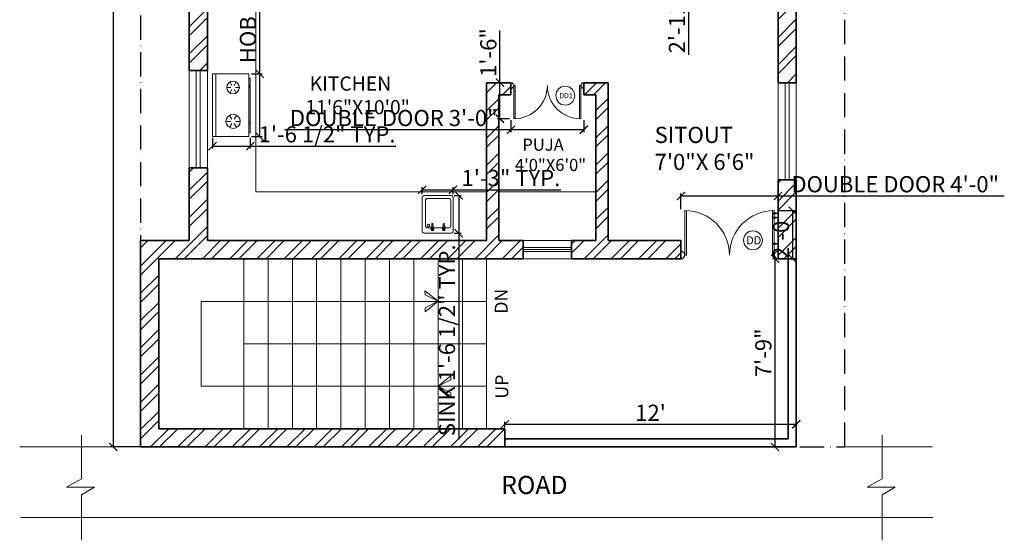
# Model space of a CAD drawing. Units: inches. Extents: x -15 to 1053, y -1 to 793.
# Tile 4 of 8: x 559 to 1046, y -1 to 256. Entities that reach past the tile are written whole.
import ezdxf

# ---------------------------------------------------------------- set-up
doc = ezdxf.new("R2010")
doc.units = ezdxf.units.IN
doc.linetypes.add('ACAD_ISO10W100', pattern=[18, 12, -3, 0, -3])
for name, color, linetype, lineweight in [('00 FURNITURE', 15, 'Continuous', 15), ('A-ANNO-DIMS', 2, 'Continuous', 18), ('A-ANNO-SYMB', 2, 'Continuous', 18), ('A-ANNO-TEXT', 7, 'Continuous', 18), ('A-AREA-IDEN', 7, 'Continuous', 18), ('A-DOOR', 4, 'Continuous', 18), ('A-FLOR-CASE', 5, 'Continuous', 18), ('A-FLOR-FIXT', 8, 'Continuous', 13), ('A-FLOR-STRS', 3, 'Continuous', 18), ('A-GLAZ', 4, 'Continuous', 18), ('A-WALL', 7, 'Continuous', 35), ('A-WALL-PATT', 8, 'Continuous', 13), ('C-PROP', 1, 'ACAD_ISO10W100', 25), ('C-ROAD', 7, 'Continuous', 18)]:
    doc.layers.add(name, color=color, linetype=linetype, lineweight=lineweight)
doc.layers.add('FURN3D', color=229, linetype='Continuous', lineweight=5, true_color=0x4a3f41)
doc.styles.add('1-100DIM', font='txt', dxfattribs={"height": 0.3})
doc.styles.get("Standard").update_dxf_attribs({"font": 'arial.ttf'})
doc.dimstyles.new('ISO-25', dxfattribs={"dimtxt": 8, "dimasz": 4, "dimexe": 1.25, "dimexo": 0.625, "dimtad": 1, "dimdec": 0, "dimlunit": 4, "dimtxsty": 'Standard', "dimblk": 'ARCHTICK', "dimcen": 3, "dimadec": 0, "dimazin": 0, "dimtfac": 1, "dimtdec": 0, "dimtmove": 0, "dimatfit": 3, "dimldrblk": 'ARCHTICK', "dimfxl": 1, "dimarcsym": 0})

# ---------------------------------------------------------------- blocks, each defined once
blk = doc.blocks.new('A$C03CC5C65')
at = {"layer": 'FURN3D'}
for p, q in [((0, 0.9, -49.92), (0, 17.82, -49.92)), ((0, 0.9, -29.27), (0, 17.82, -48.65)), ((0, 17.82, -29.27), (0, 0.9, -48.65)), ((1.56, 18.72, -49.92), (13.66, 18.72, -49.92)), ((4.37, 16.77, -25.9), (4.37, 16.84, -25.9)), ((4.37, 16.77, -25.9), (4.73, 16.4, -25.9)), ((4.37, 15.7, -25.9), (4.73, 16.12, -25.9)), ((4.37, 15.64, -25.9), (4.73, 16.06, -25.9)), ((4.37, 15.64, -25.9), (4.37, 15.7, -25.9)), ((4.48, 16.95, -25.9), (4.87, 16.59, -25.9)), ((4.48, 16.89, -25.9), (4.48, 16.95, -25.9)), ((4.48, 16.89, -25.9), (4.87, 16.52, -25.9)), ((4.48, 15.53, -25.9), (4.87, 15.89, -25.9)), ((4.63, 16.87, -25.9), (4.63, 16.8, -25.9)), ((4.63, 15.67, -25.9), (4.68, 15.67, -25.9)), ((4.63, 15.67), (4.68, 15.67)), ((4.64, 16.49, -25.9), (4.66, 16.05, -25.9)), ((4.83, 16.98, -25.9), (4.68, 16.76, -25.9)), ((4.68, 15.71, -25.9), (4.75, 14.17, -25.9)), ((4.87, 16.91, -25.9), (4.73, 16.71, -25.9)), ((5.24, 16.98, -25.9), (4.83, 16.98, -25.9)), ((4.87, 16.91, -25.9), (4.83, 16.98, -25.9)), ((5.21, 16.91, -25.9), (4.87, 16.91, -25.9)), ((5.21, 16.91, -25.9), (5.24, 16.98, -25.9)), ((5.6, 16.95, -25.9), (5.21, 16.59, -25.9)), ((5.21, 16.91, -25.9), (5.34, 16.71, -25.9)), ((5.6, 16.88, -25.9), (5.21, 16.52, -25.9)), ((5.6, 15.52, -25.9), (5.21, 15.89, -25.9)), ((5.24, 16.98, -25.9), (5.39, 16.76, -25.9)), ((5.39, 15.71, -25.9), (5.32, 14.17, -25.9)), ((5.71, 16.77, -25.9), (5.35, 16.4, -25.9)), ((5.71, 15.7, -25.9), (5.35, 16.12, -25.9)), ((5.71, 15.64, -25.9), (5.35, 16.06, -25.9)), ((5.39, 15.67, -25.9), (5.44, 15.67, -25.9)), ((5.39, 15.67), (5.44, 15.67)), ((5.43, 16.49, -25.9), (5.41, 16.05, -25.9)), ((5.44, 16.87, -25.9), (5.44, 16.8, -25.9)), ((5.6, 16.95, -25.9), (5.6, 16.88, -25.9)), ((5.6, 16.95, -25.9), (5.6, 16.88, -25.9)), ((5.71, 16.77, -25.9), (5.71, 16.83, -25.9)), ((5.71, 15.64, -25.9), (5.71, 15.7, -25.9)), ((9.98, 15.69, -25.9), (10.34, 16.11, -25.9)), ((9.98, 15.63, -25.9), (10.34, 16.05, -25.9)), ((9.98, 15.63, -25.9), (9.98, 15.69, -25.9)), ((9.99, 16.76, -25.9), (9.99, 16.83, -25.9)), ((9.99, 16.76, -25.9), (10.34, 16.39, -25.9)), ((10.09, 16.94, -25.9), (10.48, 16.58, -25.9)), ((10.09, 16.88, -25.9), (10.09, 16.94, -25.9)), ((10.09, 16.88, -25.9), (10.48, 16.51, -25.9)), ((10.09, 15.52, -25.9), (10.48, 15.88, -25.9)), ((10.25, 16.86, -25.9), (10.25, 16.8, -25.9)), ((10.25, 15.66, -25.9), (10.3, 15.66, -25.9)), ((10.25, 15.66), (10.3, 15.66)), ((10.26, 16.47, -25.9), (10.28, 16.03, -25.9)), ((10.45, 16.97, -25.9), (10.3, 16.75, -25.9)), ((10.3, 15.7, -25.9), (10.37, 14.16, -25.9)), ((10.49, 16.9, -25.9), (10.35, 16.7, -25.9)), ((10.86, 16.97, -25.9), (10.45, 16.97, -25.9)), ((10.49, 16.9, -25.9), (10.45, 16.97, -25.9)), ((10.82, 16.9, -25.9), (10.49, 16.9, -25.9)), ((10.82, 16.9, -25.9), (10.86, 16.97, -25.9)), ((11.22, 16.94, -25.9), (10.82, 16.58, -25.9)), ((10.82, 16.9, -25.9), (10.96, 16.7, -25.9)), ((11.22, 16.88, -25.9), (10.82, 16.51, -25.9)), ((11.21, 15.51, -25.9), (10.82, 15.88, -25.9)), ((10.86, 16.97, -25.9), (11.01, 16.75, -25.9)), ((11.01, 15.7, -25.9), (10.93, 14.16, -25.9)), ((11.32, 16.76, -25.9), (10.96, 16.39, -25.9)), ((11.32, 15.69, -25.9), (10.96, 16.11, -25.9)), ((11.32, 15.63, -25.9), (10.96, 16.05, -25.9)), ((11.01, 15.66, -25.9), (11.06, 15.66, -25.9)), ((11.01, 15.66), (11.06, 15.66)), ((11.05, 16.47, -25.9), (11.03, 16.03, -25.9)), ((11.06, 16.86, -25.9), (11.06, 16.8, -25.9)), ((11.22, 16.94, -25.9), (11.22, 16.88, -25.9)), ((11.22, 16.94, -25.9), (11.22, 16.88, -25.9)), ((11.32, 16.76, -25.9), (11.32, 16.83, -25.9)), ((11.32, 15.63, -25.9), (11.32, 15.69, -25.9)), ((15.22, 0.9, -29.27), (15.22, 17.82, -48.65)), ((15.22, 17.82, -29.27), (15.22, 0.9, -48.65)), ((1.56, 0, -28), (13.66, 0, -28))]:
    blk.add_line(p, q, dxfattribs=at)
at = {"layer": 'FURN3D', "elevation": -25.9}
for points in [[(1.61, 15.14), (1.62, 2.5)], [(4.66, 16.1), (2.57, 16.1)], [(10.28, 16.11), (5.41, 16.1)], [(13.12, 16.11), (11.03, 16.11)], [(14.1, 2.52), (14.09, 15.15)], [(2.58, 1.55), (13.13, 1.56)]]:
    blk.add_lwpolyline(points, dxfattribs=at)
at = {"layer": 'FURN3D'}
for centre, radius in [((3.1, 14.9, -25.9), 0.593), ((5.04, 16.22, -25.9), 0.218), ((5.04, 16.87), 0.203), ((5.04, 16.87, -25.9), 0.203), ((10.65, 16.22, -25.9), 0.218), ((10.65, 16.86), 0.203), ((10.65, 16.86, -25.9), 0.203)]:
    blk.add_circle(centre, radius, dxfattribs=at)
at = {"layer": 'FURN3D', "extrusion": (0, 0.814703, 0.579878)}
for centre, start, end in [((-1.56, -49.97, -13.7), 270, 0), ((-13.66, -49.97, -13.7), 180, 270), ((-1.56, -24.37, -16.24), 0, 90), ((-13.66, -24.37, -16.24), 90, 180)]:
    blk.add_arc(centre, 1.56, start, end, dxfattribs=at)
at = {"layer": 'FURN3D', "extrusion": (2.9e-15, -0.814703, 0.579878)}
for centre, start, end in [((1.56, -13.52, -31.49), 90, 180), ((1.56, -39.11, -28.95), 180, 270)]:
    blk.add_arc(centre, 1.56, start, end, dxfattribs=at)
at = {"layer": 'FURN3D'}
for centre, radius, start, end in [((2.6, 15.1, -25.9), 0.997, 88.2299, 182.3676), ((4.6, 16.73, -25.9), 0.252, 118.1078, 154.1122), ((4.6, 16.66, -25.9), 0.252, 118.1078, 154.1122), ((4.6, 15.75, -25.9), 0.252, 205.7141, 241.7184), ((5.04, 16.87, -25.9), 0.655, 359.2227, 180.6036), ((5.04, 16.88, -25.9), 0.655, 190.8582, 233.614), ((5.04, 16.87, -25.9), 0.406, 359.9131, 179.9131), ((4.54, 16.23, -25.9), 0.25, 317.2189, 42.6074), ((4.54, 16.29, -25.9), 0.25, 317.2189, 352.664), ((5.04, 16.6, -25.9), 0.312, 19.462, 160.6639), ((5.04, 16.24, -25.9), 0.218, 356.8132, 183.0131), ((5.04, 16.77, -25.9), 0.25, 227.2092, 312.6171), ((5.04, 16.71, -25.9), 0.25, 227.2092, 312.6171), ((5.04, 15.7, -25.9), 0.25, 47.2092, 132.6171), ((5.04, 16.44, -25.9), 0.187, 40.218, 139.6082), ((5.53, 16.23, -25.9), 0.25, 137.2189, 222.6074), ((5.53, 16.29, -25.9), 0.25, 187.1622, 222.6074), ((5.04, 16.88, -25.9), 0.655, 306.2123, 348.968), ((5.48, 16.72, -25.9), 0.252, 25.7141, 61.7184), ((5.48, 16.66, -25.9), 0.252, 25.7141, 61.7184), ((5.48, 15.75, -25.9), 0.252, 298.1078, 334.1122), ((10.21, 15.74, -25.9), 0.252, 205.7141, 241.7184), ((10.21, 16.72, -25.9), 0.252, 118.1078, 154.1122), ((10.21, 16.65, -25.9), 0.252, 118.1078, 154.1122), ((10.65, 16.86, -25.9), 0.655, 359.2227, 180.6036), ((10.65, 16.86, -25.9), 0.655, 190.8582, 233.614), ((10.65, 16.86, -25.9), 0.406, 359.9131, 179.9131), ((10.16, 16.22, -25.9), 0.25, 317.2189, 42.6074), ((10.16, 16.28, -25.9), 0.25, 317.2189, 352.664), ((10.66, 16.59, -25.9), 0.312, 19.462, 160.6639), ((10.65, 16.23, -25.9), 0.218, 356.8132, 183.0131), ((10.65, 16.7, -25.9), 0.25, 227.2092, 312.6171), ((10.65, 15.69, -25.9), 0.25, 47.2092, 132.6171), ((10.65, 16.76, -25.9), 0.25, 227.2092, 312.6171), ((10.65, 16.44, -25.9), 0.187, 40.218, 139.6082), ((11.15, 16.22, -25.9), 0.25, 137.2189, 222.6074), ((11.15, 16.28, -25.9), 0.25, 187.1622, 222.6074), ((10.65, 16.86, -25.9), 0.655, 306.2123, 348.968), ((11.1, 15.74, -25.9), 0.252, 298.1078, 334.1122), ((11.1, 16.72, -25.9), 0.252, 25.7141, 61.7184), ((11.1, 16.65, -25.9), 0.252, 25.7141, 61.7184), ((13.09, 15.11, -25.9), 0.997, 357.7426, 91.8802), ((5.04, 14.37, -25.9), 0.298, 194.8671, 343.5351), ((5.03, 14.18, -25.9), 0.281, 182.7661, 357.0602), ((10.65, 14.36, -25.9), 0.298, 194.8671, 343.5351), ((10.65, 14.17, -25.9), 0.281, 182.7661, 357.0602), ((2.61, 2.54, -25.9), 0.997, 177.7426, 271.8802), ((13.1, 2.55, -25.9), 0.997, 268.2299, 2.3676)]:
    blk.add_arc(centre, radius, start, end, dxfattribs=at)
at = {"layer": 'FURN3D', "extrusion": (-2.9e-15, -0.814703, 0.579878)}
for centre, start, end in [((13.66, -13.52, -31.49), 0, 90), ((13.66, -39.11, -28.95), 270, 0)]:
    blk.add_arc(centre, 1.56, start, end, dxfattribs=at)
blk = doc.blocks.new('_ArchTick')
at = {"color": 0, "linetype": 'ByBlock', "const_width": 0.15}
blk.add_lwpolyline([(-0.5, -0.5), (0.5, 0.5)], dxfattribs=at)
blk = doc.blocks.new('*D19')
at = {"layer": 'A-ANNO-DIMS', "color": 0, "lineweight": -2, "transparency": 16777216}
for p, q in [((618.45, 764.76), (604.32, 764.76)), ((605.57, 764.76), (605.57, 44.76)), ((618.45, 44.76), (604.32, 44.76))]:
    blk.add_line(p, q, dxfattribs=at)
at = {"layer": 'Defpoints', "color": 0, "transparency": 16777216}
for p in [(619.07, 764.76), (605.57, 44.76), (619.07, 44.76)]:
    blk.add_point(p, dxfattribs=at)
at = {"layer": 'A-ANNO-DIMS', "color": 0, "lineweight": -2, "transparency": 16777216, "xscale": 4, "yscale": 4, "zscale": 4}
for p, rotation in [((605.57, 764.76), 90), ((605.57, 44.76), 270)]:
    blk.add_blockref('_ArchTick', p, dxfattribs=dict(at, rotation=rotation))
at = {"layer": 'A-ANNO-DIMS', "color": 0, "transparency": 16777216, "insert": (600.86, 404.76), "char_height": 8, "attachment_point": 5, "rotation": 90}
blk.add_mtext("60'", dxfattribs=at)
blk = doc.blocks.new('A$C21540130')
at = {"layer": 'FURN3D'}
for p, q in [((1.57, 0), (1.57, 31.11)), ((9.61, 25.31), (8.63, 27.01)), ((10.79, 25.31), (11.77, 27.01)), ((9.02, 24.29, -27.54), (7.06, 24.29, -27.54)), ((9.61, 23.27), (8.63, 21.57)), ((10.79, 23.27), (11.77, 21.57)), ((11.38, 24.29, -27.54), (13.34, 24.29, -27.54)), ((9.61, 8.56), (8.43, 10.6)), ((10.79, 8.56), (11.97, 10.6)), ((9.02, 7.54), (6.67, 7.54)), ((9.61, 6.52), (8.43, 4.48)), ((10.79, 6.52), (11.97, 4.48)), ((11.38, 7.54), (13.73, 7.54))]:
    blk.add_line(p, q, dxfattribs=at)
for points in [[(0, 0), (0, 31.11), (17.9, 31.11), (17.9, 0)], [(18.68, 1.96), (18.68, 28.83), (17.9, 28.83), (17.9, 1.96)]]:
    blk.add_lwpolyline(points, close=True, dxfattribs=at)
for centre, radius in [((10.2, 24.29), 3.14), ((10.2, 7.54), 3.53)]:
    blk.add_circle(centre, radius, dxfattribs=at)
for points in [[(17.9, 24.03), (18.29, 24.03), (17.9, 25.6), (18.29, 25.6)], [(17.9, 6.05), (18.29, 6.05), (17.9, 7.62), (18.29, 7.62)]]:
    blk.add_solid(points, dxfattribs=at)
blk = doc.blocks.new('PUJA')
at = {"layer": '00 FURNITURE'}
for p, q in [((-1940.35, -16093.35), (-1958.14, -16093.35)), ((-1940.35, -16093.93), (-1958.13, -16093.93)), ((-1941.8, -16091.75), (-1938.89, -16091.75)), ((-1941.8, -16092.33), (-1941.8, -16091.75)), ((-1941.22, -16092.62), (-1941.51, -16092.62)), ((-1940.35, -16093.35), (-1940.35, -16093.93)), ((-1939.18, -16092.62), (-1939.47, -16092.62)), ((-1938.89, -16091.75), (-1938.89, -16092.33)), ((-1940.35, -16128.93), (-1958.14, -16128.93)), ((-1940.35, -16128.35), (-1958.13, -16128.35)), ((-1941.8, -16129.96), (-1941.8, -16130.54)), ((-1941.22, -16129.66), (-1941.51, -16129.66)), ((-1940.35, -16128.93), (-1940.35, -16128.35)), ((-1939.18, -16129.66), (-1939.47, -16129.66)), ((-1938.89, -16130.54), (-1938.89, -16129.96)), ((-1941.8, -16130.54), (-1938.89, -16130.54))]:
    blk.add_line(p, q, dxfattribs=at)
for points in [[(-1939.47, -16092.62), (-1939.47, -16092.91, -0.414214), (-1939.76, -16093.21), (-1940.93, -16093.21, -0.414214), (-1941.22, -16092.91), (-1941.22, -16092.62)], [(-1939.47, -16129.66), (-1939.47, -16129.37, 0.414214), (-1939.76, -16129.08), (-1940.93, -16129.08, 0.414214), (-1941.22, -16129.37), (-1941.22, -16129.66)]]:
    blk.add_lwpolyline(points, format="xyb", dxfattribs=at)
for centre, radius, start, end in [((-1940.35, -16093.35), 17.79, 180, 270), ((-1941.51, -16092.33), 0.292, 180, 270), ((-1939.18, -16092.33), 0.292, 270, 0), ((-1940.35, -16128.93), 17.79, 90, 180), ((-1941.51, -16129.96), 0.292, 90, 180), ((-1939.18, -16129.96), 0.292, 0, 90)]:
    blk.add_arc(centre, radius, start, end, dxfattribs=at)
blk = doc.blocks.new('*D28')
at = {"layer": 'A-ANNO-DIMS', "color": 0, "lineweight": -2, "transparency": 16777216}
for p, q in [((799.07, 54.39), (799.07, 57.2)), ((799.07, 55.95), (943.07, 55.95)), ((943.07, 45.39), (943.07, 57.2))]:
    blk.add_line(p, q, dxfattribs=at)
at = {"layer": 'Defpoints', "color": 0, "transparency": 16777216}
for p in [(799.07, 53.76), (943.07, 55.95), (943.07, 44.76)]:
    blk.add_point(p, dxfattribs=at)
at = {"layer": 'A-ANNO-DIMS', "color": 0, "lineweight": -2, "transparency": 16777216, "xscale": 4, "yscale": 4, "zscale": 4, "rotation": 180}
blk.add_blockref('_ArchTick', (799.07, 55.95), dxfattribs=at)
at = {"layer": 'A-ANNO-DIMS', "color": 0, "lineweight": -2, "transparency": 16777216, "xscale": 4, "yscale": 4, "zscale": 4}
blk.add_blockref('_ArchTick', (943.07, 55.95), dxfattribs=at)
at = {"layer": 'A-ANNO-DIMS', "color": 0, "transparency": 16777216, "insert": (871.07, 60.59), "char_height": 8, "attachment_point": 5}
blk.add_mtext("12'", dxfattribs=at)
blk = doc.blocks.new('*D29')
at = {"layer": 'A-ANNO-DIMS', "color": 0, "lineweight": -2, "transparency": 16777216}
for p, q in [((942.45, 137.76), (931.3, 137.76)), ((932.55, 137.76), (932.55, 44.76)), ((942.45, 44.76), (931.3, 44.76))]:
    blk.add_line(p, q, dxfattribs=at)
at = {"layer": 'Defpoints', "color": 0, "transparency": 16777216}
for p in [(943.07, 137.76), (932.55, 44.76), (943.07, 44.76)]:
    blk.add_point(p, dxfattribs=at)
at = {"layer": 'A-ANNO-DIMS', "color": 0, "lineweight": -2, "transparency": 16777216, "xscale": 4, "yscale": 4, "zscale": 4}
for p, rotation in [((932.55, 137.76), 90), ((932.55, 44.76), 270)]:
    blk.add_blockref('_ArchTick', p, dxfattribs=dict(at, rotation=rotation))
at = {"layer": 'A-ANNO-DIMS', "color": 0, "transparency": 16777216, "insert": (927.84, 91.26), "char_height": 8, "attachment_point": 5, "rotation": 90}
blk.add_mtext('7\'-9"', dxfattribs=at)
blk = doc.blocks.new('BREAK-SYMBOL')
for p, q in [((7.31, 51.97), (7.31, 30.42)), ((7.31, 30.42), (0, 26.2)), ((0, 26.2), (13.84, 26.2)), ((13.84, 26.2), (7.31, 22.43)), ((7.31, 22.43), (7.31, 0))]:
    blk.add_line(p, q)
blk = doc.blocks.new('*D47')
at = {"layer": 'A-ANNO-DIMS', "color": 0, "lineweight": -2, "transparency": 16777216}
for p, q in [((894.42, 333.87), (888.54, 333.87)), ((889.79, 333.87), (889.79, 298.84)), ((894.42, 298.84), (888.54, 298.84)), ((889.79, 298.84), (889.79, 238.47))]:
    blk.add_line(p, q, dxfattribs=at)
at = {"layer": 'Defpoints', "color": 0, "transparency": 16777216}
for p in [(895.05, 333.87), (889.79, 298.84), (895.05, 298.84)]:
    blk.add_point(p, dxfattribs=at)
at = {"layer": 'A-ANNO-DIMS', "color": 0, "lineweight": -2, "transparency": 16777216, "xscale": 4, "yscale": 4, "zscale": 4}
for p, rotation in [((889.79, 333.87), 90), ((889.79, 298.84), 270)]:
    blk.add_blockref('_ArchTick', p, dxfattribs=dict(at, rotation=rotation))
at = {"layer": 'A-ANNO-DIMS', "color": 0, "transparency": 16777216, "insert": (885.15, 266.65), "char_height": 8, "attachment_point": 5, "rotation": 90}
blk.add_mtext('2\'-11" TYP.', dxfattribs=at)
blk = doc.blocks.new('*D48')
at = {"layer": 'A-ANNO-DIMS', "color": 0, "lineweight": -2, "transparency": 16777216}
for p, q in [((774.07, 169.08), (777.51, 169.08)), ((776.26, 169.08), (776.26, 150.36)), ((774.07, 150.36), (777.51, 150.36)), ((776.26, 150.36), (776.26, 48.55))]:
    blk.add_line(p, q, dxfattribs=at)
at = {"layer": 'Defpoints', "color": 0, "transparency": 16777216}
for p in [(773.45, 169.08), (773.45, 150.36), (776.26, 150.36)]:
    blk.add_point(p, dxfattribs=at)
at = {"layer": 'A-ANNO-DIMS', "color": 0, "lineweight": -2, "transparency": 16777216, "xscale": 4, "yscale": 4, "zscale": 4}
for p, rotation in [((776.26, 169.08), 90), ((776.26, 150.36), 270)]:
    blk.add_blockref('_ArchTick', p, dxfattribs=dict(at, rotation=rotation))
at = {"layer": 'A-ANNO-DIMS', "color": 0, "transparency": 16777216, "insert": (771.5, 97.45), "char_height": 8, "attachment_point": 5, "rotation": 90}
blk.add_mtext('SINK 1\'-6 1/2" TYP.', dxfattribs=at)
blk = doc.blocks.new('*D49')
at = {"layer": 'A-ANNO-DIMS', "color": 0, "lineweight": -2, "transparency": 16777216}
for p, q in [((758.23, 169.7), (758.23, 173.13)), ((758.23, 171.88), (773.45, 171.88)), ((773.45, 169.7), (773.45, 173.13)), ((773.45, 171.88), (826.71, 171.88))]:
    blk.add_line(p, q, dxfattribs=at)
at = {"layer": 'Defpoints', "color": 0, "transparency": 16777216}
for p in [(773.45, 171.88), (758.23, 169.08), (773.45, 169.08)]:
    blk.add_point(p, dxfattribs=at)
at = {"layer": 'A-ANNO-DIMS', "color": 0, "lineweight": -2, "transparency": 16777216, "xscale": 4, "yscale": 4, "zscale": 4, "rotation": 180}
blk.add_blockref('_ArchTick', (758.23, 171.88), dxfattribs=at)
at = {"layer": 'A-ANNO-DIMS', "color": 0, "lineweight": -2, "transparency": 16777216, "xscale": 4, "yscale": 4, "zscale": 4}
blk.add_blockref('_ArchTick', (773.45, 171.88), dxfattribs=at)
at = {"layer": 'A-ANNO-DIMS', "color": 0, "transparency": 16777216, "insert": (802.08, 176.6), "char_height": 8, "attachment_point": 5}
blk.add_mtext('1\'-3" TYP.', dxfattribs=at)
blk = doc.blocks.new('*D50')
at = {"layer": 'A-ANNO-DIMS', "color": 0, "lineweight": -2, "transparency": 16777216}
for p, q in [((677.95, 229.2), (677.95, 310.11)), ((673.9, 229.2), (679.2, 229.2)), ((677.95, 198.09), (677.95, 229.2)), ((673.9, 198.09), (679.2, 198.09))]:
    blk.add_line(p, q, dxfattribs=at)
at = {"layer": 'Defpoints', "color": 0, "transparency": 16777216}
for p in [(673.28, 229.2), (677.95, 229.2), (673.28, 198.09)]:
    blk.add_point(p, dxfattribs=at)
at = {"layer": 'A-ANNO-DIMS', "color": 0, "lineweight": -2, "transparency": 16777216, "xscale": 4, "yscale": 4, "zscale": 4}
for p, rotation in [((677.95, 229.2), 90), ((677.95, 198.09), 270)]:
    blk.add_blockref('_ArchTick', p, dxfattribs=dict(at, rotation=rotation))
at = {"layer": 'A-ANNO-DIMS', "color": 0, "transparency": 16777216, "insert": (673.18, 271.65), "char_height": 8, "attachment_point": 5, "rotation": 90}
blk.add_mtext('HOB 2\'-7" TYP.', dxfattribs=at)
blk = doc.blocks.new('*D51')
at = {"layer": 'A-ANNO-DIMS', "color": 0, "lineweight": -2, "transparency": 16777216}
for p, q in [((654.6, 197.47), (654.6, 192.18)), ((673.28, 197.47), (673.28, 192.18)), ((654.6, 193.43), (673.28, 193.43)), ((673.28, 193.43), (745.18, 193.43))]:
    blk.add_line(p, q, dxfattribs=at)
at = {"layer": 'Defpoints', "color": 0, "transparency": 16777216}
for p in [(654.6, 198.09), (673.28, 198.09), (673.28, 193.43)]:
    blk.add_point(p, dxfattribs=at)
at = {"layer": 'A-ANNO-DIMS', "color": 0, "lineweight": -2, "transparency": 16777216, "xscale": 4, "yscale": 4, "zscale": 4, "rotation": 180}
blk.add_blockref('_ArchTick', (654.6, 193.43), dxfattribs=at)
at = {"layer": 'A-ANNO-DIMS', "color": 0, "lineweight": -2, "transparency": 16777216, "xscale": 4, "yscale": 4, "zscale": 4}
blk.add_blockref('_ArchTick', (673.28, 193.43), dxfattribs=at)
at = {"layer": 'A-ANNO-DIMS', "color": 0, "transparency": 16777216, "insert": (711.23, 198.19), "char_height": 8, "attachment_point": 5}
blk.add_mtext('1\'-6 1/2" TYP.', dxfattribs=at)
blk = doc.blocks.new('*D54')
at = {"layer": 'A-ANNO-DIMS', "color": 0, "lineweight": -2, "transparency": 16777216}
for p, q in [((886.07, 162.21), (886.07, 170.03)), ((886.07, 168.78), (934.07, 168.78)), ((934.07, 162.21), (934.07, 170.03)), ((934.07, 168.78), (1045.89, 168.78))]:
    blk.add_line(p, q, dxfattribs=at)
at = {"layer": 'Defpoints', "color": 0, "transparency": 16777216}
for p in [(934.07, 168.78), (886.07, 161.58), (934.07, 161.58)]:
    blk.add_point(p, dxfattribs=at)
at = {"layer": 'A-ANNO-DIMS', "color": 0, "lineweight": -2, "transparency": 16777216, "xscale": 4, "yscale": 4, "zscale": 4, "rotation": 180}
blk.add_blockref('_ArchTick', (886.07, 168.78), dxfattribs=at)
at = {"layer": 'A-ANNO-DIMS', "color": 0, "lineweight": -2, "transparency": 16777216, "xscale": 4, "yscale": 4, "zscale": 4}
blk.add_blockref('_ArchTick', (934.07, 168.78), dxfattribs=at)
at = {"layer": 'A-ANNO-DIMS', "color": 0, "transparency": 16777216, "insert": (991.98, 173.55), "char_height": 8, "attachment_point": 5}
blk.add_mtext('DOUBLE DOOR 4\'-0"', dxfattribs=at)
blk = doc.blocks.new('*D55')
at = {"layer": 'A-ANNO-DIMS', "color": 0, "lineweight": -2, "transparency": 16777216}
for p, q in [((934.7, 161.58), (942.52, 161.58)), ((941.27, 161.58), (941.27, 137.76)), ((934.7, 137.76), (942.52, 137.76))]:
    blk.add_line(p, q, dxfattribs=at)
at = {"layer": 'Defpoints', "color": 0, "transparency": 16777216}
for p in [(934.07, 161.58), (934.07, 137.76), (941.27, 137.76)]:
    blk.add_point(p, dxfattribs=at)
at = {"layer": 'A-ANNO-DIMS', "color": 0, "lineweight": -2, "transparency": 16777216, "xscale": 4, "yscale": 4, "zscale": 4}
for p, rotation in [((941.27, 161.58), 90), ((941.27, 137.76), 270)]:
    blk.add_blockref('_ArchTick', p, dxfattribs=dict(at, rotation=rotation))
at = {"layer": 'A-ANNO-DIMS', "color": 0, "transparency": 16777216, "insert": (936.56, 149.67), "char_height": 8, "attachment_point": 5, "rotation": 90}
blk.add_mtext('2\'-0"', dxfattribs=at)
blk = doc.blocks.new('*D56')
at = {"layer": 'A-ANNO-DIMS', "color": 0, "lineweight": -2, "transparency": 16777216}
for p, q in [((802.07, 206.27), (802.07, 200.25)), ((838.07, 206.27), (838.07, 200.25)), ((802.07, 201.5), (690.26, 201.5)), ((838.07, 201.5), (802.07, 201.5))]:
    blk.add_line(p, q, dxfattribs=at)
at = {"layer": 'Defpoints', "color": 0, "transparency": 16777216}
for p in [(802.07, 206.9), (838.07, 206.9), (802.07, 201.5)]:
    blk.add_point(p, dxfattribs=at)
at = {"layer": 'A-ANNO-DIMS', "color": 0, "lineweight": -2, "transparency": 16777216, "xscale": 4, "yscale": 4, "zscale": 4}
for p, rotation in [((802.07, 201.5), 180.0000000034012), ((838.07, 201.5), 3.4012793e-09)]:
    blk.add_blockref('_ArchTick', p, dxfattribs=dict(at, rotation=rotation))
at = {"layer": 'A-ANNO-DIMS', "color": 0, "transparency": 16777216, "insert": (744.17, 206.27), "char_height": 8, "attachment_point": 5, "rotation": 0}
blk.add_mtext('DOUBLE DOOR 3\'-0"', dxfattribs=at)
blk = doc.blocks.new('*D57')
at = {"layer": 'A-ANNO-DIMS', "color": 0, "lineweight": -2, "transparency": 16777216}
for p, q in [((796.67, 224.76), (796.67, 250.53)), ((801.45, 224.76), (795.42, 224.76)), ((796.67, 206.9), (796.67, 224.76)), ((801.45, 206.9), (795.42, 206.9))]:
    blk.add_line(p, q, dxfattribs=at)
at = {"layer": 'Defpoints', "color": 0, "transparency": 16777216}
for p in [(796.67, 224.76), (802.07, 224.76), (802.07, 206.9)]:
    blk.add_point(p, dxfattribs=at)
at = {"layer": 'A-ANNO-DIMS', "color": 0, "lineweight": -2, "transparency": 16777216, "xscale": 4, "yscale": 4, "zscale": 4}
for p, rotation in [((796.67, 224.76), 90), ((796.67, 206.9), 270)]:
    blk.add_blockref('_ArchTick', p, dxfattribs=dict(at, rotation=rotation))
at = {"layer": 'A-ANNO-DIMS', "color": 0, "transparency": 16777216, "insert": (791.96, 239.65), "char_height": 8, "attachment_point": 5, "rotation": 90}
blk.add_mtext('1\'-6"', dxfattribs=at)

msp = doc.modelspace()

# ---------------------------------------------------------------- hatches: boundary and pattern name
at = {"layer": 'A-WALL-PATT'}
h = msp.add_hatch(dxfattribs=at)
h.set_pattern_fill('ANSI32', color=256)
h.paths.add_polyline_path([(754.07, 502.76), (754.07, 503.76), (652.07, 503.76), (652.07, 593.76), (643.07, 593.76), (643.07, 485.76), (652.07, 485.76), (652.07, 497.76), (754.07, 497.76)])
h.paths.add_polyline_path([(754.07, 449.76), (730.07, 449.76), (730.07, 467.76), (724.07, 467.76), (724.07, 449.76), (652.07, 449.76), (652.07, 461.76), (643.07, 461.76), (643.07, 374.76), (652.07, 374.76), (652.07, 443.76), (754.07, 443.76)])
h.paths.add_polyline_path([(757.07, 740.76), (643.07, 740.76), (643.07, 641.76), (652.07, 641.76), (652.07, 731.76), (700.07, 731.76), (700.07, 701.76), (706.07, 701.76), (706.07, 731.76), (757.07, 731.76)])
h.paths.add_polyline_path([(943.07, 740.76), (781.07, 740.76), (781.07, 731.76), (790.07, 731.76), (790.07, 671.76), (688.07, 671.76), (688.07, 665.76), (790.07, 665.76), (790.07, 497.76), (796.07, 497.76), (796.07, 502.76), (796.07, 731.76), (844.07, 731.76), (844.07, 701.76), (850.07, 701.76), (850.07, 731.76), (934.07, 731.76), (934.07, 713.76), (943.07, 713.76)])
h.paths.add_polyline_path([(943.07, 689.76), (934.07, 689.76), (934.07, 671.76), (832.07, 671.76), (832.07, 665.76), (934.07, 665.76), (934.07, 608.76), (943.07, 608.76)], flags=17)
h.paths.add_polyline_path([(943.07, 560.76), (934.07, 560.76), (934.07, 503.76), (832.07, 503.76), (832.07, 497.76), (934.07, 497.76), (934.07, 488.76), (943.07, 488.76)])
h.paths.add_polyline_path([(796.07, 449.76), (790.07, 449.76), (790.07, 444.76), (790.07, 326.76), (643.07, 326.76), (643.07, 320.76), (724.07, 320.76), (724.07, 266.76), (730.07, 266.76), (730.07, 320.76), (790.07, 320.76), (790.07, 272.76), (760.07, 272.76), (760.07, 266.76), (796.07, 266.76)])
h.paths.add_polyline_path([(652.07, 266.76), (688.07, 266.76), (688.07, 271.76), (688.07, 272.76), (643.07, 272.76), (643.07, 230.76), (652.07, 230.76)])
h.paths.add_polyline_path([(652.07, 182.76), (643.07, 182.76), (643.07, 146.76), (619.07, 146.76), (619.07, 44.76), (799.07, 44.76), (799.07, 53.76), (628.07, 53.76), (628.07, 137.76), (808.07, 137.76), (808.07, 146.76), (796.07, 146.76), (796.07, 218.76), (802.07, 218.76), (802.07, 224.76), (790.07, 224.76), (790.07, 146.76), (652.07, 146.76)])
h.paths.add_polyline_path([(886.07, 141.37), (886.07, 146.76), (850.07, 146.76), (850.07, 224.76), (838.07, 224.76), (838.07, 222.06), (838.07, 218.76), (844.07, 218.76), (844.07, 146.76), (832.07, 146.76), (832.07, 137.76), (886.07, 137.76)])
h.paths.add_polyline_path([(943.07, 176.76), (934.07, 176.76), (934.07, 137.76), (943.07, 137.76)])
h.paths.add_polyline_path([(943.07, 440.76), (934.07, 440.76), (934.07, 224.76), (943.07, 224.76)])

# ---------------------------------------------------------------- linework, layer by layer
at = {"layer": 'A-ANNO-TEXT'}
for centre in [(828.93, 218.35), (921.67, 146.87)]:
    msp.add_circle(centre, 4.67, dxfattribs=at)
at = {"layer": 'A-FLOR-CASE'}
for p, q in [((676.07, 266.76), (676.07, 170.76)), ((676.07, 170.76), (790.07, 170.76)), ((796.07, 170.76), (844.07, 170.76))]:
    msp.add_line(p, q, dxfattribs=at)
at = {"layer": 'A-FLOR-STRS'}
for p, q in [((670.07, 137.76), (670.07, 53.76)), ((682.07, 137.76), (682.07, 53.76)), ((694.07, 137.76), (694.07, 53.76)), ((706.07, 137.76), (706.07, 53.76)), ((718.07, 137.76), (718.07, 53.76)), ((730.07, 137.76), (730.07, 53.76)), ((742.07, 137.76), (742.07, 53.76)), ((754.07, 137.76), (754.07, 53.76)), ((766.07, 137.76), (766.07, 53.76)), ((778.07, 137.76), (778.07, 53.76)), ((790.07, 137.76), (790.07, 53.76)), ((670.07, 95.76), (790.07, 95.76)), ((766.07, 74.76), (772.46, 69.56)), ((772.46, 71.55), (766.07, 74.76)), ((772.46, 69.56), (772.46, 71.55))]:
    msp.add_line(p, q, dxfattribs=at)
for points in [[(759.64, 119.88), (766.07, 116.76), (759.61, 121.87)], [(759.74, 113.46), (766.07, 116.76), (759.76, 111.47)], [(772.46, 79.96), (772.46, 77.97), (766.07, 74.76)]]:
    msp.add_lwpolyline(points, close=True, dxfattribs=at)
msp.add_lwpolyline([(790.07, 74.76), (649.07, 74.76), (649.07, 116.7), (790.07, 116.7)], dxfattribs=at)
at = {"layer": 'A-GLAZ'}
for p, q in [((643.07, 230.76), (643.07, 182.76)), ((646.57, 230.76), (646.57, 182.76)), ((648.57, 230.76), (648.57, 182.76)), ((652.07, 230.76), (652.07, 182.76)), ((934.07, 224.76), (934.07, 176.76)), ((937.57, 224.76), (937.57, 176.76)), ((939.57, 224.76), (939.57, 176.76)), ((943.07, 224.76), (943.07, 176.76)), ((832.07, 143.26), (808.07, 143.26)), ((832.07, 142.26), (808.07, 142.26)), ((832.07, 141.26), (808.07, 141.26))]:
    msp.add_line(p, q, dxfattribs=at)
msp.add_lwpolyline([(808.07, 146.76), (808.07, 137.76), (832.07, 137.76), (832.07, 146.76)], close=True, dxfattribs=at)
at = {"layer": 'A-WALL'}
for p, q in [((934.07, 224.76), (934.07, 440.76)), ((943.07, 224.76), (943.07, 440.76)), ((643.07, 272.76), (643.07, 230.76)), ((652.07, 266.76), (652.07, 230.76)), ((652.07, 230.76), (643.07, 230.76)), ((790.07, 224.76), (802.07, 224.76)), ((790.07, 224.76), (790.07, 146.76)), ((802.07, 218.76), (802.07, 224.76)), ((838.07, 218.76), (838.07, 224.76)), ((838.07, 224.76), (850.07, 224.76)), ((850.07, 224.76), (850.07, 146.76)), ((934.07, 224.76), (943.07, 224.76)), ((796.07, 218.76), (802.07, 218.76)), ((796.07, 218.76), (796.07, 146.76)), ((838.07, 218.76), (844.07, 218.76)), ((844.07, 218.76), (844.07, 146.76)), ((652.07, 182.76), (643.07, 182.76)), ((643.07, 182.76), (643.07, 146.76)), ((652.07, 182.76), (652.07, 146.76)), ((934.07, 137.76), (934.07, 176.76)), ((934.07, 176.76), (943.07, 176.76)), ((943.07, 137.76), (943.07, 176.76)), ((619.07, 146.76), (643.07, 146.76)), ((619.07, 146.76), (619.07, 44.76)), ((652.07, 146.76), (790.07, 146.76)), ((796.07, 146.76), (808.07, 146.76)), ((808.07, 146.76), (808.07, 137.76)), ((832.07, 146.76), (832.07, 137.76)), ((832.07, 146.76), (844.07, 146.76)), ((850.07, 146.76), (886.07, 146.76)), ((886.07, 137.76), (886.07, 146.76)), ((628.07, 137.76), (808.07, 137.76)), ((628.07, 137.76), (628.07, 53.76)), ((832.07, 137.76), (886.07, 137.76)), ((934.07, 137.76), (943.07, 137.76)), ((939.07, 137.76), (939.07, 48.76)), ((943.07, 137.76), (943.07, 44.76)), ((628.07, 53.76), (799.07, 53.76)), ((799.07, 53.76), (799.07, 44.76)), ((799.07, 48.76), (939.07, 48.76)), ((619.07, 44.76), (799.07, 44.76)), ((799.07, 44.76), (943.07, 44.76))]:
    msp.add_line(p, q, dxfattribs=at)
at = {"layer": 'C-PROP'}
for p, q in [((619.07, 764.76), (619.07, 44.76)), ((967.07, 44.76), (967.07, 764.76)), ((619.07, 44.76), (967.07, 44.76))]:
    msp.add_line(p, q, dxfattribs=at)
at = {"layer": 'C-ROAD'}
for p, q in [((619.07, 44.76), (559.32, 44.76)), ((967.07, 44.76), (1010.42, 44.76)), ((559.95, 9.83), (1010.56, 9.83))]:
    msp.add_line(p, q, dxfattribs=at)

# ---------------------------------------------------------------- block references
at = {"layer": 'A-ANNO-SYMB'}
for p in [(582.51, -1.39), (978.17, -1.39)]:
    msp.add_blockref('BREAK-SYMBOL', p, dxfattribs=at)
at = {"layer": 'A-DOOR'}
for p, xscale, yscale, zscale, rotation in [((-14131.62, 2024.12), 0.928034371616032, 0.928034371616032, 0.928034371616032, 90.00000000340147), ((20845.67, -2261.38), 1.237379162154587, 1.237379162154587, 1.237379162154587, 270.0000000034012)]:
    msp.add_blockref('PUJA', p, dxfattribs=dict(at, xscale=xscale, yscale=yscale, zscale=zscale, rotation=rotation))
at = {"layer": 'A-FLOR-FIXT'}
msp.add_blockref('A$C21540130', (654.6, 198.09), dxfattribs=at)
at = {"layer": 'A-FLOR-FIXT', "xscale": -1, "rotation": 180}
msp.add_blockref('A$C03CC5C65', (758.23, 169.08, 49.92), dxfattribs=at)

# ---------------------------------------------------------------- texts
at = {"layer": 'A-ANNO-TEXT', "attachment_point": 1}
for s, width, insert, char_height in [('DD1', 8.4888, (825.99, 219.6), 2.5), ('DD', 8.4888, (918.29, 148.88), 4), ('ROAD', 36.3273, (797.25, 30.45), 9)]:
    msp.add_mtext_dynamic_manual_height_columns(s, width=width, gutter_width=12.5, heights=[0], dxfattribs=dict(at, insert=insert, char_height=char_height))
at = {"layer": 'A-ANNO-TEXT', "char_height": 6.4099, "attachment_point": 3, "rotation": 90, "style": '1-100DIM'}
for s, insert in [('\\pxqc;{\\f@Malgun Gothic|b0|i0|c0|p34;DN}', (794.06, 139.01)), ('\\pxqc;{\\f@Malgun Gothic|b0|i0|c0|p34;UP}', (794.35, 96.8))]:
    msp.add_mtext_dynamic_manual_height_columns(s, width=44.4859, gutter_width=15.85, heights=[0], dxfattribs=dict(at, insert=insert))
at = {"layer": 'A-AREA-IDEN', "insert": (696.22, 227.83), "char_height": 7, "attachment_point": 1, "style": '1-100DIM'}
msp.add_mtext_dynamic_manual_height_columns('{\\f@Malgun Gothic|b0|i0|c0|p34;   KITCHEN\\P  11\'6"X10\'0"}', width=99.7063, gutter_width=15.85, heights=[0], dxfattribs=at)
at = {"layer": 'A-AREA-IDEN', "attachment_point": 1}
for s, width, heights, insert, char_height in [('  SITOUT\\P  7\'0"X 6\'6"', 62.9334, [0], (868.19, 202.95), 8), ('      PUJA       \\P    4\'0"X6\'0"', 44.0107, [18.97], (796.73, 197.11), 6)]:
    msp.add_mtext_dynamic_manual_height_columns(s, width=width, gutter_width=12.5, heights=heights, dxfattribs=dict(at, insert=insert, char_height=char_height))

# ---------------------------------------------------------------- dimensions: what is measured, and where the dimension line sits
at = {"layer": 'A-ANNO-DIMS'}
for base, p1, p2, angle, override, picture, middle in [((605.57, 44.76), (619.07, 764.76), (619.07, 44.76), 90, {"dimclrd": 0, "dimclre": 0, "dimclrt": 0}, '*D19', (600.86, 404.76)), ((796.67, 224.76), (802.07, 206.9), (802.07, 224.76), 90, {"dimdec": 1, "dimrnd": 0, "dimzin": 1, "dimlunit": 4, "dimfrac": 2}, '*D57', (791.96, 239.65)), ((941.27, 137.76), (934.07, 161.58), (934.07, 137.76), 270, {"dimdec": 1, "dimrnd": 0, "dimzin": 1, "dimlunit": 4, "dimfrac": 2}, '*D55', (936.56, 149.67)), ((932.55, 44.76), (943.07, 137.76), (943.07, 44.76), 90, {"dimclrd": 0, "dimclre": 0, "dimclrt": 0}, '*D29', (927.84, 91.26))]:
    dim = msp.add_linear_dim(base=base, p1=p1, p2=p2, angle=angle, dimstyle='ISO-25', override=override, dxfattribs=at)
    dim.commit()
    dim.dimension.update_dxf_attribs({"geometry": picture, "text_midpoint": middle})
for base, p1, p2, angle, text, picture, middle in [((889.79, 298.84), (895.05, 333.87), (895.05, 298.84), 270, '<> TYP.', '*D47', (885.15, 266.65)), ((677.95, 229.2), (673.28, 198.09), (673.28, 229.2), 90, 'HOB <> TYP.', '*D50', (673.18, 271.65)), ((802.07, 201.5), (838.07, 206.9), (802.07, 206.9), 180, 'DOUBLE DOOR <>', '*D56', (744.17, 206.27)), ((934.07, 168.78), (886.07, 161.58), (934.07, 161.58), 0, 'DOUBLE DOOR <>', '*D54', (991.98, 173.55)), ((776.26, 150.36), (773.45, 169.08), (773.45, 150.36), 270, 'SINK <> TYP.', '*D48', (771.5, 97.45))]:
    dim = msp.add_linear_dim(base=base, p1=p1, p2=p2, angle=angle, text=text, dimstyle='ISO-25', override={"dimdec": 1, "dimrnd": 0, "dimzin": 1, "dimlunit": 4, "dimfrac": 2}, dxfattribs=at)
    dim.commit()
    dim.dimension.update_dxf_attribs({"geometry": picture, "text_midpoint": middle})
for base, p1, p2, picture, middle in [((673.28, 193.43), (654.6, 198.09), (673.28, 198.09), '*D51', (711.23, 198.19)), ((773.45, 171.88), (758.23, 169.08), (773.45, 169.08), '*D49', (802.08, 176.6))]:
    dim = msp.add_linear_dim(base=base, p1=p1, p2=p2, text='<> TYP.', dimstyle='ISO-25', override={"dimdec": 1, "dimrnd": 0, "dimzin": 1, "dimlunit": 4, "dimfrac": 2}, dxfattribs=at)
    dim.commit()
    dim.dimension.update_dxf_attribs({"geometry": picture, "text_midpoint": middle})
dim = msp.add_linear_dim(base=(943.07, 55.95), p1=(799.07, 53.76), p2=(943.07, 44.76), dimstyle='ISO-25', override={"dimclrd": 0, "dimclre": 0, "dimclrt": 0}, dxfattribs=at)
dim.commit()
dim.dimension.update_dxf_attribs({"geometry": '*D28', "text_midpoint": (871.07, 60.59)})

doc.saveas('drawing.dxf')
